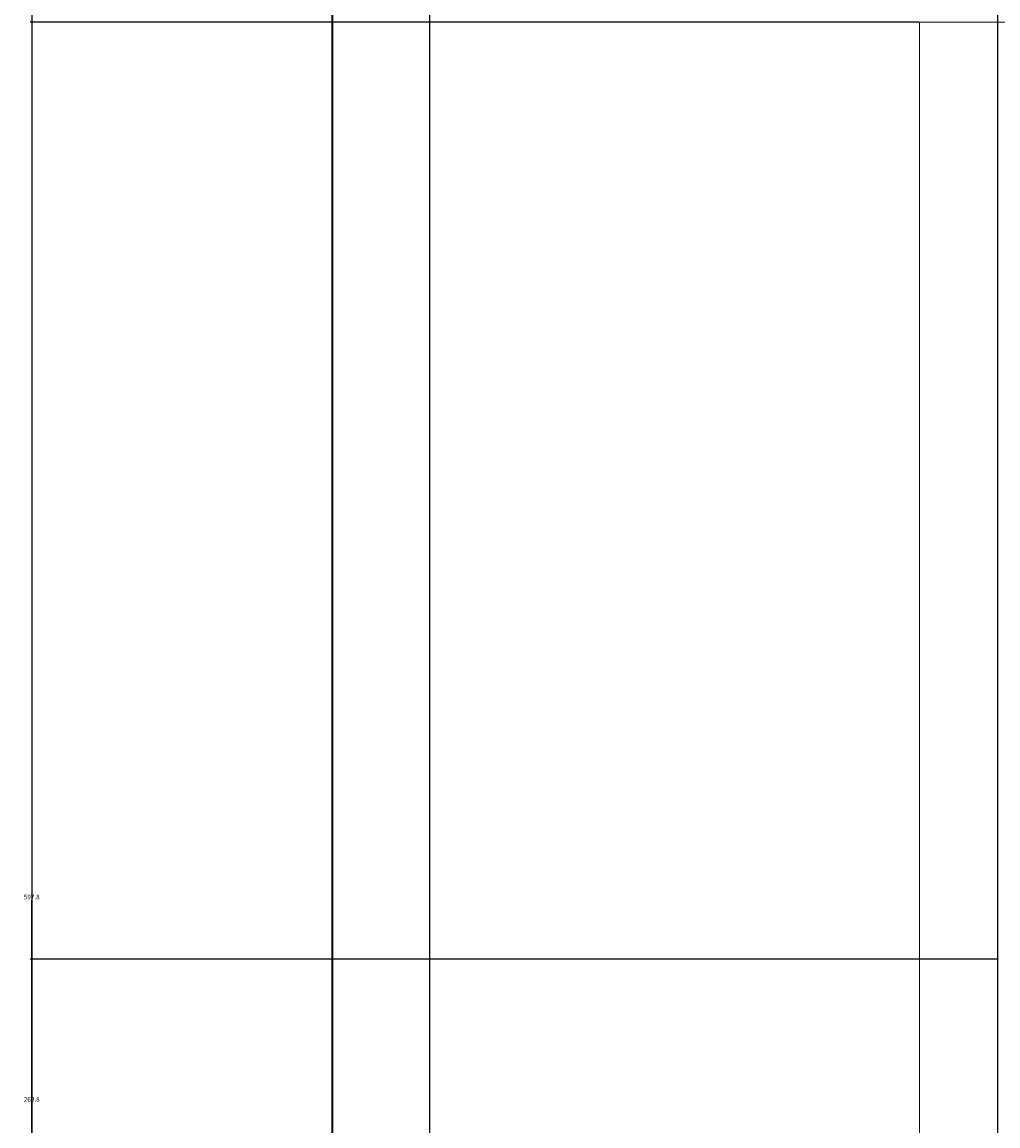
# Model space of a CAD drawing. Units: inches. Extents: x -26 to 776, y -22 to 650.
# Tile 11 of 62: x -26 to 92, y 287 to 420. Entities that reach past the tile are written whole.
import ezdxf

# ---------------------------------------------------------------- set-up
doc = ezdxf.new("R2010")
doc.units = ezdxf.units.IN
doc.header["$MEASUREMENT"] = 0
for name, color, linetype, lineweight in [('A-ANNO-DIMS', 2, 'Continuous', 18), ('A-WALL', 7, 'Continuous', 35), ('A-WALL-TRIM', 7, 'Continuous', 18)]:
    doc.layers.add(name, color=color, linetype=linetype, lineweight=lineweight)
doc.styles.get("Standard").update_dxf_attribs({"font": 'arial.ttf'})
doc.dimstyles.get("Standard").update_dxf_attribs({"dimtxt": 0.5625, "dimasz": 0.18, "dimexe": 0.18, "dimexo": 0.0625, "dimgap": 0.09, "dimtad": 0, "dimtih": 1, "dimtoh": 1, "dimdec": 4, "dimzin": 0, "dimdsep": 46, "dimlunit": 4, "dimtxsty": 'Standard', "dimcen": 0.09, "dimadec": 0, "dimazin": 0, "dimtfac": 1, "dimtdec": 4, "dimtofl": 0, "dimtmove": 0, "dimatfit": 3, "dimfxl": 1, "dimtolj": 1, "dimtzin": 0, "dimarcsym": 0})

# ---------------------------------------------------------------- blocks, each defined once
blk = doc.blocks.new('*D14')
at = {"layer": 'A-ANNO-DIMS', "color": 0, "lineweight": -2, "transparency": 16777216}
for p, q in [((191.62, 613.27), (-25.48, 613.27)), ((-25.3, 613.09), (-25.3, 314.75)), ((-25.3, 15.66), (-25.3, 314)), ((11.04, 15.48), (-25.48, 15.48))]:
    blk.add_line(p, q, dxfattribs=at)
at = {"layer": 'A-ANNO-DIMS', "color": 0, "transparency": 16777216}
for points in [[(-25.33, 613.09), (-25.27, 613.09), (-25.3, 613.27)], [(-25.33, 15.66), (-25.27, 15.66), (-25.3, 15.48)]]:
    blk.add_solid(points, dxfattribs=at)
at = {"layer": 'Defpoints', "color": 0, "transparency": 16777216}
for p in [(-25.3, 613.27), (191.68, 613.27), (11.11, 15.48)]:
    blk.add_point(p, dxfattribs=at)
at = {"layer": 'A-ANNO-DIMS', "color": 0, "transparency": 16777216, "insert": (-25.3, 314.38), "char_height": 0.562, "attachment_point": 5}
blk.add_mtext('\\A1;597.8', dxfattribs=at)
blk = doc.blocks.new('*D22')
at = {"layer": 'A-ANNO-DIMS', "color": 0, "lineweight": -2, "transparency": 16777216}
for p, q in [((22.89, 15.33), (22.89, 649.86)), ((23.07, 649.68), (119.19, 649.68)), ((217.77, 649.68), (121.65, 649.68)), ((217.95, 15.54), (217.95, 649.86))]:
    blk.add_line(p, q, dxfattribs=at)
at = {"layer": 'A-ANNO-DIMS', "color": 0, "transparency": 16777216}
for points in [[(23.07, 649.71), (23.07, 649.65), (22.89, 649.68)], [(217.77, 649.71), (217.77, 649.65), (217.95, 649.68)]]:
    blk.add_solid(points, dxfattribs=at)
at = {"layer": 'Defpoints', "color": 0, "transparency": 16777216}
for p in [(217.95, 649.68), (22.89, 15.27), (217.95, 15.48)]:
    blk.add_point(p, dxfattribs=at)
at = {"layer": 'A-ANNO-DIMS', "color": 0, "transparency": 16777216, "insert": (120.42, 649.68), "char_height": 0.562, "attachment_point": 5}
blk.add_mtext('\\A1;195.06', dxfattribs=at)
blk = doc.blocks.new('*D24')
at = {"layer": 'A-ANNO-DIMS', "color": 0, "lineweight": -2, "transparency": 16777216}
for p, q in [((11.11, 15.54), (11.11, 649.86)), ((11.29, 649.68), (15.77, 649.68)), ((22.71, 649.68), (18.23, 649.68)), ((22.89, 15.33), (22.89, 649.86))]:
    blk.add_line(p, q, dxfattribs=at)
at = {"layer": 'A-ANNO-DIMS', "color": 0, "transparency": 16777216}
for points in [[(11.29, 649.71), (11.29, 649.65), (11.11, 649.68)], [(22.71, 649.71), (22.71, 649.65), (22.89, 649.68)]]:
    blk.add_solid(points, dxfattribs=at)
at = {"layer": 'Defpoints', "color": 0, "transparency": 16777216}
for p in [(22.89, 649.68), (11.11, 15.48), (22.89, 15.27)]:
    blk.add_point(p, dxfattribs=at)
at = {"layer": 'A-ANNO-DIMS', "color": 0, "transparency": 16777216, "insert": (17, 649.68), "char_height": 0.562, "attachment_point": 5}
blk.add_mtext('\\A1;11.782', dxfattribs=at)
blk = doc.blocks.new('*D25')
at = {"layer": 'A-ANNO-DIMS', "color": 0, "lineweight": -2, "transparency": 16777216}
for p, q in [((11.11, 221.7), (11.11, 649.86)), ((11.29, 649.68), (50.34, 649.68)), ((91.46, 649.68), (52.41, 649.68)), ((91.64, 271.37), (91.64, 649.86))]:
    blk.add_line(p, q, dxfattribs=at)
at = {"layer": 'A-ANNO-DIMS', "color": 0, "transparency": 16777216}
for points in [[(11.29, 649.71), (11.29, 649.65), (11.11, 649.68)], [(91.46, 649.71), (91.46, 649.65), (91.64, 649.68)]]:
    blk.add_solid(points, dxfattribs=at)
at = {"layer": 'Defpoints', "color": 0, "transparency": 16777216}
for p in [(91.64, 649.68), (91.64, 271.31), (11.11, 221.64)]:
    blk.add_point(p, dxfattribs=at)
at = {"layer": 'A-ANNO-DIMS', "color": 0, "transparency": 16777216, "insert": (51.38, 649.68), "char_height": 0.562, "attachment_point": 5}
blk.add_mtext('\\A1;80.54', dxfattribs=at)
blk = doc.blocks.new('*D27')
at = {"layer": 'A-ANNO-DIMS', "color": 0, "lineweight": -2, "transparency": 16777216}
for p, q in [((91.58, 306.86), (-25.48, 306.86)), ((-25.3, 306.68), (-25.3, 239.79)), ((-25.3, 172.15), (-25.3, 239.04)), ((91.58, 171.97), (-25.48, 171.97))]:
    blk.add_line(p, q, dxfattribs=at)
at = {"layer": 'A-ANNO-DIMS', "color": 0, "transparency": 16777216}
for points in [[(-25.33, 306.68), (-25.27, 306.68), (-25.3, 306.86)], [(-25.33, 172.15), (-25.27, 172.15), (-25.3, 171.97)]]:
    blk.add_solid(points, dxfattribs=at)
at = {"layer": 'Defpoints', "color": 0, "transparency": 16777216}
for p in [(-25.3, 306.86), (91.64, 306.86), (91.64, 171.97)]:
    blk.add_point(p, dxfattribs=at)
at = {"layer": 'A-ANNO-DIMS', "color": 0, "transparency": 16777216, "insert": (-25.3, 239.41), "char_height": 0.562, "attachment_point": 5}
blk.add_mtext('\\A1;134.88', dxfattribs=at)
blk = doc.blocks.new('*D36')
at = {"layer": 'A-ANNO-DIMS', "color": 0, "lineweight": -2, "transparency": 16777216}
for p, q in [((82.07, 420.28), (-25.48, 420.28)), ((-25.3, 420.1), (-25.3, 290.26)), ((-25.3, 159.66), (-25.3, 289.5)), ((82.07, 159.48), (-25.48, 159.48))]:
    blk.add_line(p, q, dxfattribs=at)
at = {"layer": 'A-ANNO-DIMS', "color": 0, "transparency": 16777216}
for points in [[(-25.33, 420.1), (-25.27, 420.1), (-25.3, 420.28)], [(-25.33, 159.66), (-25.27, 159.66), (-25.3, 159.48)]]:
    blk.add_solid(points, dxfattribs=at)
at = {"layer": 'Defpoints', "color": 0, "transparency": 16777216}
for p in [(-25.3, 420.28), (82.13, 420.28), (82.13, 159.48)]:
    blk.add_point(p, dxfattribs=at)
at = {"layer": 'A-ANNO-DIMS', "color": 0, "transparency": 16777216, "insert": (-25.3, 289.88), "char_height": 0.562, "attachment_point": 5}
blk.add_mtext('\\A1;260.8', dxfattribs=at)

msp = doc.modelspace()

# ---------------------------------------------------------------- linework, layer by layer
at = {"layer": 'A-WALL'}
for p, q in [((11.1074, 338.1203), (11.1074, 458.1203)), ((11.1074, 159.4824), (11.1074, 338.1203))]:
    msp.add_line(p, q, dxfattribs=at)
at = {"layer": 'A-WALL-TRIM'}
msp.add_lwpolyline([(82.134, 159.4824), (209.091, 159.4824), (209.091, 420.2783), (82.134, 420.2783)], close=True, dxfattribs=at)

# ---------------------------------------------------------------- dimensions: what is measured, and where the dimension line sits
at = {"layer": 'A-ANNO-DIMS'}
for base, p1, p2, override, picture, middle in [((22.8891, 649.6763), (11.1074, 15.4824), (22.8891, 15.2701), {"dimdec": 3, "dimlfac": 1, "dimrnd": 0, "dimzin": 0, "dimdsep": 46, "dimlunit": 2}, '*D24', (16.9982, 649.6763)), ((91.6448, 649.6763), (11.1074, 221.6413), (91.6448, 271.3091), {"dimdec": 2, "dimlfac": 1, "dimrnd": 0, "dimzin": 0, "dimdsep": 46, "dimlunit": 2}, '*D25', (51.3761, 649.6763)), ((217.9529, 649.6763), (22.8891, 15.2701), (217.9529, 15.4824), {"dimdec": 2, "dimlfac": 1, "dimrnd": 0, "dimzin": 0, "dimdsep": 46, "dimlunit": 2}, '*D22', (120.421, 649.6763))]:
    dim = msp.add_linear_dim(base=base, p1=p1, p2=p2, dimstyle='Standard', override=override, dxfattribs=at)
    dim.commit()
    dim.dimension.update_dxf_attribs({"geometry": picture, "text_midpoint": middle})
for base, p1, p2, override, picture, middle in [((-25.2976, 613.2713), (11.1074, 15.4824), (191.6782, 613.2713), {"dimdec": 1, "dimlfac": 1, "dimrnd": 0, "dimzin": 0, "dimdsep": 46, "dimlunit": 2}, '*D14', (-25.2976, 314.3769)), ((-25.2976, 420.2783), (82.134, 159.4824), (82.134, 420.2783), {"dimdec": 1, "dimlfac": 1, "dimrnd": 0, "dimzin": 0, "dimdsep": 46, "dimlunit": 2}, '*D36', (-25.2976, 289.8803)), ((-25.2976, 306.8552), (91.6448, 171.9734), (91.6448, 306.8552), {"dimdec": 2, "dimlfac": 1, "dimrnd": 0, "dimzin": 0, "dimdsep": 46, "dimlunit": 2}, '*D27', (-25.2976, 239.4143))]:
    dim = msp.add_linear_dim(base=base, p1=p1, p2=p2, angle=90, dimstyle='Standard', override=override, dxfattribs=at)
    dim.commit()
    dim.dimension.update_dxf_attribs({"geometry": picture, "text_midpoint": middle})

doc.saveas('drawing.dxf')
